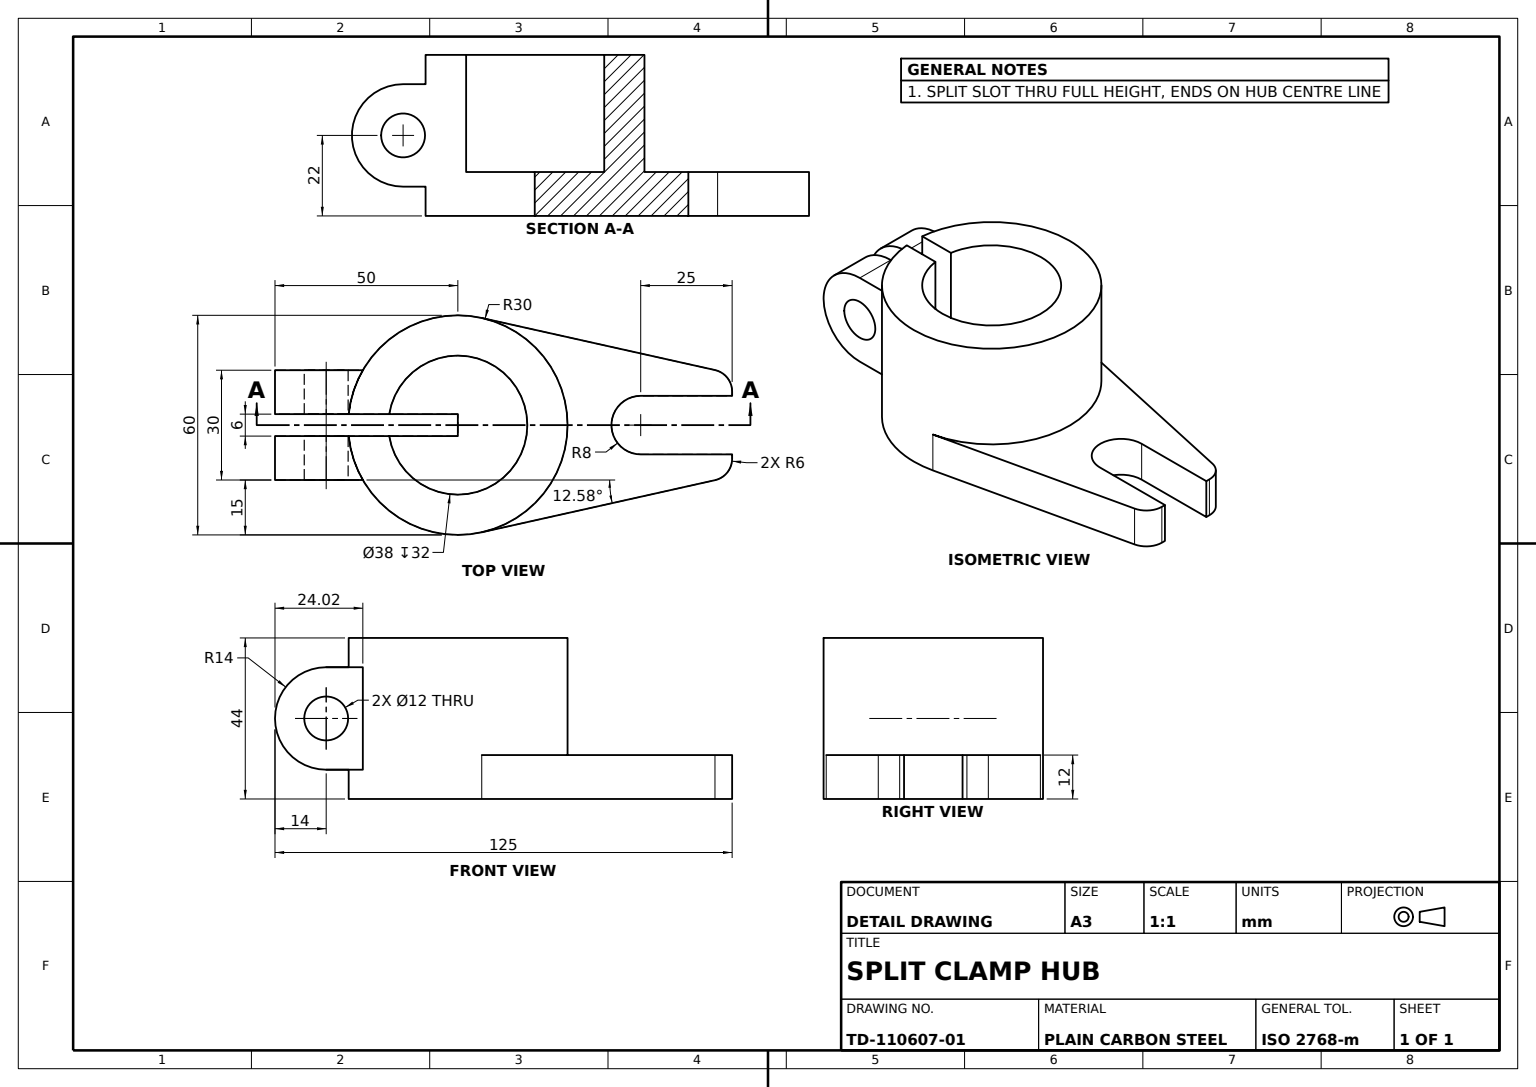
from build123d import *

# Parameters (mm, degrees)
BASE_FLANGE_DEPTH      = 12
SPLIT_CLAMP_RING_DEPTH = 32
CLAMP_EAR_A_SKETCH_R   = 6
CLAMP_EAR_A_DEPTH      = 12
CLAMP_START            = -12
CLAMP_EAR_B_SKETCH_R   = 6
CLAMP_EAR_B_DEPTH      = 12


with BuildPart() as part:
    # Base Flange Sketch → Base Flange (new body)
    with BuildSketch(Plane(origin=(0, 0, 0), x_dir=(1, 0, 0), z_dir=(0, 1, 0))):
        with BuildLine():
            Line((-29.849623113, 3), (0, 3))
            Line((0, 3), (0, -3))
            Line((0, -3), (-29.849623113, -3))
            ThreePointArc((-29.849623113, -3), (-17.565731604, -24.319643772), (6.534455825, -29.279700939))
            Line((6.534455825, -29.279700939), (70.306891165, -15.047377923))
            ThreePointArc((70.306891165, -15.047377923), (73.681951889, -12.943680599), (75, -9.191437735))
            Line((75, -9.191437735), (75, -8))
            Line((75, -8), (50, -8))
            ThreePointArc((50, -8), (42, 0), (50, 8))
            Line((50, 8), (75, 8))
            Line((75, 8), (75, 9.191437735))
            ThreePointArc((75, 9.191437735), (73.681951889, 12.943680599), (70.306891165, 15.047377923))
            Line((70.306891165, 15.047377923), (6.534455825, 29.279700939))
            ThreePointArc((6.534455825, 29.279700939), (-17.565731604, 24.319643772), (-29.849623113, 3))
        make_face()
    extrude(amount=BASE_FLANGE_DEPTH)

    # Clamp Ring Sketch → Split Clamp Ring (add)
    with BuildSketch(Plane(origin=(0, 12, 0), x_dir=(1, 0, 0), z_dir=(0, 1, 0))):
        with BuildLine():
            ThreePointArc((6.534455825, 29.279700939), (-17.565731604, 24.319643772), (-29.849623113, 3))
            Line((-29.849623113, 3), (-18.761663039, 3))
            ThreePointArc((-18.761663039, 3), (19, 0), (-18.761663039, -3))
            Line((-18.761663039, -3), (-29.849623113, -3))
            ThreePointArc((-29.849623113, -3), (-17.565731604, -24.319643772), (6.534455825, -29.279700939))
            ThreePointArc((6.534455825, -29.279700939), (30, 0), (6.534455825, 29.279700939))
        make_face()
    extrude(amount=SPLIT_CLAMP_RING_DEPTH)

    # Clamp Ear A Sketch → Clamp Ear A (add)
    with BuildSketch(Plane.XY.offset(3)):
        with BuildLine():
            Line((-36, 36), (-25, 36))
            Line((-25, 36), (-25, 8))
            Line((-25, 8), (-36, 8))
            ThreePointArc((-36, 8), (-50, 22), (-36, 36))
        make_face()
        with Locations((-36, 22)):
            Circle(CLAMP_EAR_A_SKETCH_R, mode=Mode.SUBTRACT)
    extrude(amount=CLAMP_EAR_A_DEPTH)

    # Clamp Ear B Sketch → Clamp Ear B (add)
    with BuildSketch(Plane.XY.offset(-3).offset(CLAMP_START)):
        with BuildLine():
            Line((-36, 36), (-25, 36))
            Line((-25, 36), (-25, 8))
            Line((-25, 8), (-36, 8))
            ThreePointArc((-36, 8), (-50, 22), (-36, 36))
        make_face()
        with Locations((-36, 22)):
            Circle(CLAMP_EAR_B_SKETCH_R, mode=Mode.SUBTRACT)
    extrude(amount=CLAMP_EAR_B_DEPTH)


solid = part.part
